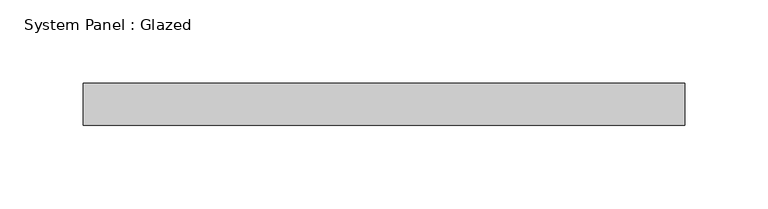
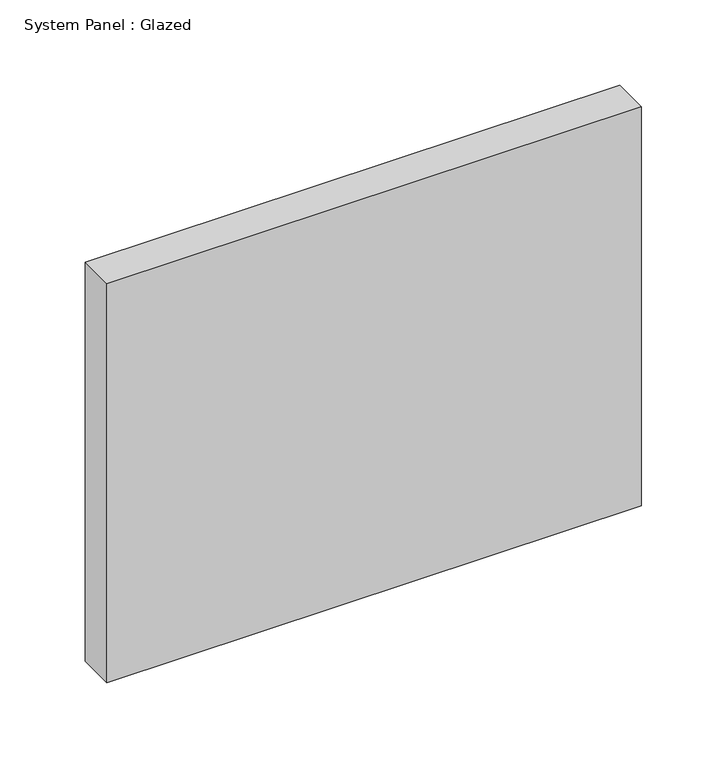
"""IFC4 building model written with IfcOpenShell, lengths in millimetres: plate geometry, System Panel : Glazed."""

from ifc_helpers import new_model, si_unit, origin, origin_with_axes, place, context, project, spatial, polyline, outline, extrude, source, transform, mapped, element, save


def system_panel_glazed_499f07c7(model_context):
    return source(origin(), model_context, "Body", "SweptSolid", [
        extrude(outline(polyline([(180.975, 19.05), (-180.975, 19.05), (-180.975, 44.45), (180.975, 44.45), (180.975, 19.05)])), origin_with_axes(), (0.0, 0.0, 1.0), 285.75),
    ])


if __name__ == "__main__":
    model = new_model("IFC4")
    model_context = context("Model", 3, world=origin())
    ifc_project = project(units=[si_unit("LENGTHUNIT", "METRE", prefix="MILLI")], contexts=[model_context])
    site = spatial("IfcSite", under=ifc_project)
    building = spatial("IfcBuilding", under=site)
    placement = place(None, origin())
    system_panel_glazed_shape = system_panel_glazed_499f07c7(model_context)
    element("IfcPlate", 1, ObjectType="System Panel : Glazed", at=placement, inside=building, context=model_context, shape_type="MappedRepresentation", body=[
        mapped(system_panel_glazed_shape, transform((0.0, 0.0, 0.0), x_axis=(1.0, 0.0, 0.0), y_axis=(0.0, 1.0, 0.0), z_axis=(0.0, 0.0, 1.0))),
    ])
    save(model, "model.ifc")

# Revit data of these elements
# Type "System Panel : Glazed"
#   Construction Type Id = "GSP4R"
#   Analytic Construction = "1/8 in Pilkington single glazing"
#   Visual Light Transmittance = 0.9
#   Solar Heat Gain Coefficient = 0.86
#   Heat Transfer Coefficient (U) = 1.18115 BTU/(h·ft²·°F)
#   Define Thermal Properties by = 1
# Element 1 (IfcPlate, "System Panel : Glazed")
#   Materials on its faces: "Glass"
# Materials
#   "Glass": class "Glass", colour RGB 0 128 192, transparency 0.75, Description = "Soda Lime Glass", Cost = 0
